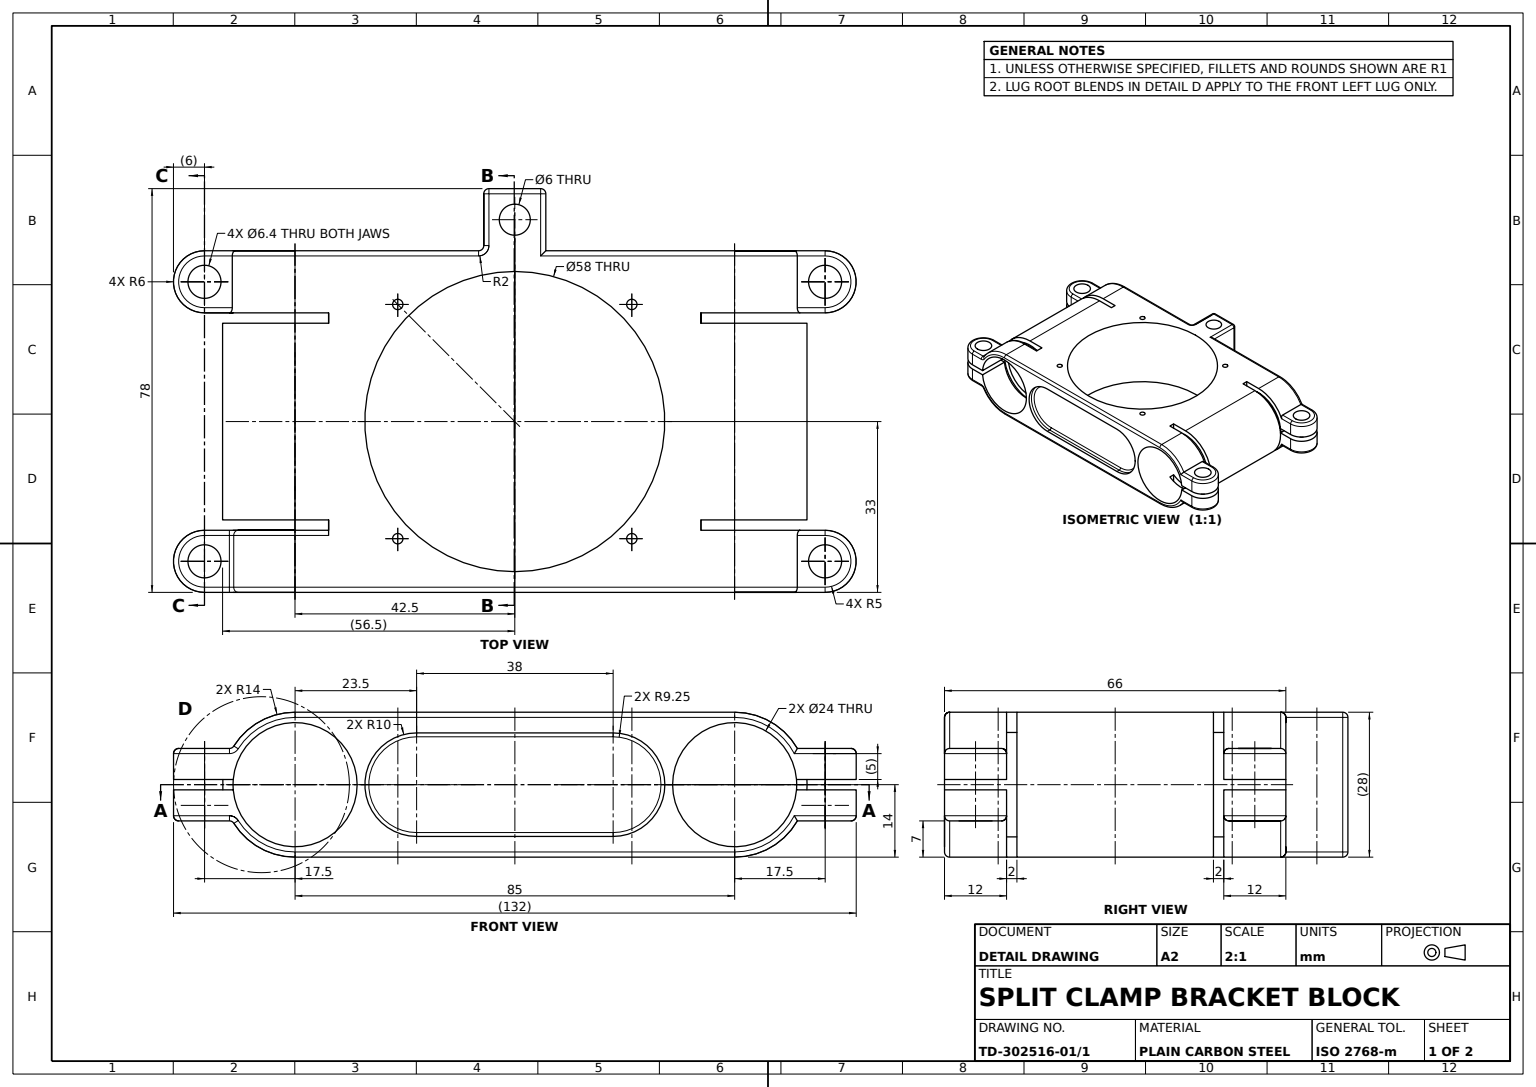
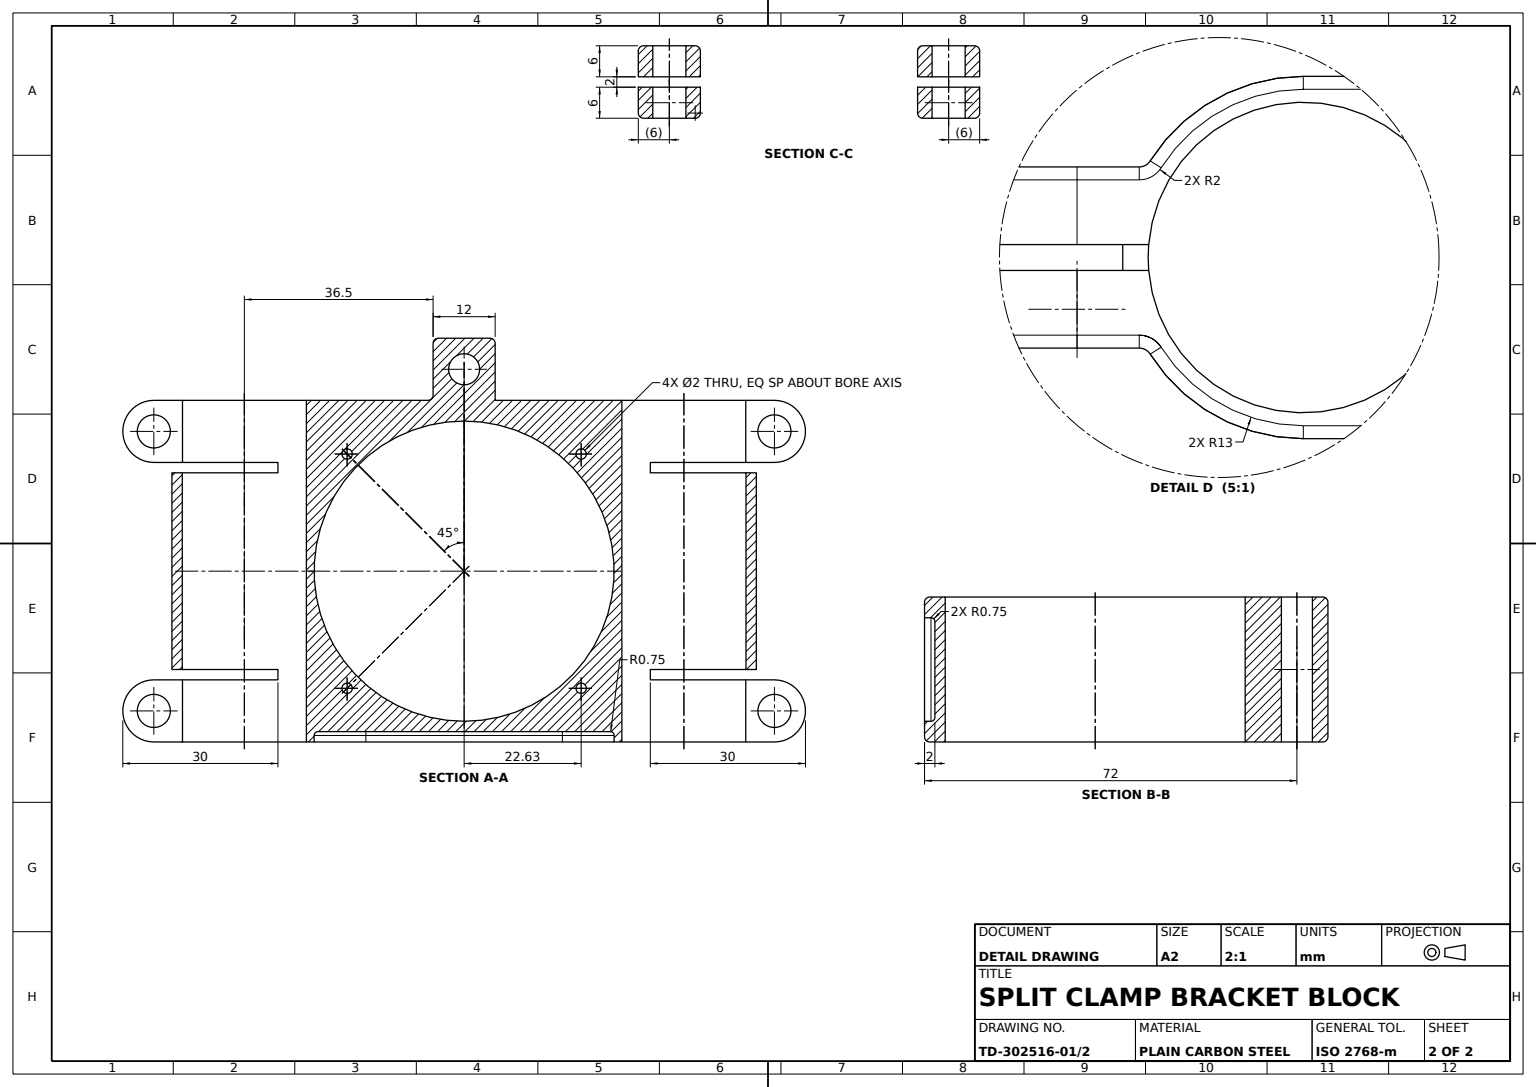
SolidWorks part; units mm, degrees
material "Plain Carbon Steel"
ref_plane "Front Plane" through (0, 0, 0) normal (0, 0, 1) x (1, 0, 0)
ref_plane "Top Plane" through (0, 0, 0) normal (0, 1, 0) x (1, 0, 0)
ref_plane "Right Plane" through (0, 0, 0) normal (1, 0, 0) x (0, 0, -1)
sketch "Body Profile Sketch" plane through (0, 0, 0) normal (0, 0, 1) x (1, 0, 0)
  line L0 (0, 0) -> (85, 0) construction
  line L1 (0, 14) -> (85, 14)
  line L2 (0, -14) -> (85, -14)
  arc A0 (0, 14) -> (0, -14) centre (0, 0) ccw
  arc A1 (85, -14) -> (85, 14) centre (85, 0) ccw
  point P3 (42.5, 0)
  dimension "D2" = 14
  dimension "D1" = 85
extrude "Carriage Body" add sketch "Body Profile Sketch" against normal blind 66
sketch "Rod Bore A Sketch" plane through (0, 0, 0) normal (0, 0, 1) x (1, 0, 0)
  circle A0 centre (0, 0) radius 12
  circle A1 centre (85, 0) radius 12
  dimension "D1" = 24
extrude "Rod Bore A Ø24" cut sketch "Rod Bore A Sketch" against normal blind 66
sketch "Side Pocket Sketch" plane through (0, 0, 0) normal (0, 0, 1) x (1, 0, 0)
  line L0 (23.5, 0) -> (61.5, 0) construction
  line L1 (23.5, 10) -> (61.5, 10)
  line L2 (23.5, -10) -> (61.5, -10)
  line L3 (85, 12) -> (85, 0) construction
  arc A0 (23.5, 10) -> (23.5, -10) centre (23.5, 0) ccw
  arc A1 (61.5, -10) -> (61.5, 10) centre (61.5, 0) ccw
  circle A2 centre (85, 0) radius 12 construction
  point P3 (42.5, 0)
  dimension "D3" = 10
  dimension "D1" = 38
  dimension "D2" = 42.5
extrude "Side Pocket 2mm" cut sketch "Side Pocket Sketch" against normal blind 2
sketch "Centre Bore Sketch" plane through (0, 14, 0) normal (0, 1, 0) x (1, 0, 0)
  line L0 (-14, 66) -> (-14, 0) construction
  circle A0 centre (42.5, 33) radius 29
  dimension "D1" = 58
  dimension "D2" = 33
  dimension "D3" = 56.5
extrude "Centre Bore Ø58" cut sketch "Centre Bore Sketch" against normal through all
sketch "Bore Screw Holes Sketch" plane through (0, 14, 0) normal (0, 1, 0) x (1, 0, 0)
  line L0 (42.5, 33) -> (68.5238, 59.0238) construction
  circle A1 centre (65.1274, 55.6274) radius 1
  circle A2 centre (65.1274, 10.3726) radius 1
  circle A3 centre (19.8726, 10.3726) radius 1
  circle A4 centre (19.8726, 55.6274) radius 1
  dimension "D1" = 22.6274
  dimension "D3" = 2
  dimension "D2" = 45
  dimension "D5" = 22.6274
  dimension "D6" = 22.6274
  dimension "D7" = 22.6274
  dimension "D4" = 4
extrude "Bore Screw Holes 4xØ2" cut sketch "Bore Screw Holes Sketch" against normal through all
ref_plane "Plane1" through (0, 0, 0) normal (0, 1, 0) x (1, 0, 0)
sketch "Clamp Lug Sketch" plane through (0, 0, 0) normal (0, 1, 0) x (1, 0, 0)
  line L0 (85, 0) -> (0, 0) construction
  line L1 (102.5, 12) -> (96.5, 12)
  line L2 (96.5, 12) -> (96.5, 0)
  line L3 (85, 0) -> (99, 0) construction
  line L4 (96.5, 0) -> (102.5, 0)
  arc A0 (102.5, 0) -> (102.5, 12) centre (102.5, 6) ccw
  dimension "D1" = 12
  dimension "D2" = 17.5
  dimension "D3" = 6
  dimension "D4" = 6
extrude "Clamp Lug" add sketch "Clamp Lug Sketch" along normal mid plane 14
sketch "Lug Split Sketch" plane through (0, 0, 0) normal (0, 1, 0) x (1, 0, 0)
  line L0 (97.1244, 0) -> (102.5, 0) construction
  line L1 (102.5, 12) -> (97.1244, 12) construction
  line L2 (97.1244, 0) -> (102.5, 0)
  line L3 (102.5, 12) -> (97.1244, 12)
  line L4 (97.1244, 12) -> (92.1244, 12)
  line L5 (92.1244, 12) -> (92.1244, 0)
  line L6 (85, 0) -> (97.1244, 0) construction
  line L7 (92.1244, 0) -> (97.1244, 0)
  arc A0 (102.5, 0) -> (102.5, 12) centre (102.5, 6) ccw construction
  arc A1 (102.5, 0) -> (102.5, 12) centre (102.5, 6) ccw
  dimension "D1" = 5
extrude "Lug Split" cut sketch "Lug Split Sketch" against normal mid plane 2
sketch "Lug Hole Sketch" plane through (0, 7, 0) normal (0, 1, 0) x (1, 0, 0)
  circle A0 centre (102.5, 6) radius 3.2
  dimension "D1" = 6.4
extrude "Lug Hole Ø6.4" cut sketch "Lug Hole Sketch" against normal through all
ref_plane "Plane2" through (0, 0, -33) normal (0, 0, 1) x (1, 0, 0)
mirror "Lug Mirror Plane2" about plane through (0, 0, -33) normal (0, 0, 1) of "Lug Split", "Lug Hole Ø6.4", "Clamp Lug"
ref_plane "Plane4" through (42.5, 0, 0) normal (1, 0, 0) x (0, 0, -1)
mirror "Lug Mirror Plane4" about plane through (42.5, 0, 0) normal (1, 0, 0) of "Lug Split", "Lug Hole Ø6.4", "Clamp Lug"
mirror "Lug Pair Mirror Plane2" about plane through (0, 0, -33) normal (0, 0, 1) of "Clamp Lug", "Lug Split", "Lug Hole Ø6.4", "Lug Mirror Plane4"
sketch "Rod Bore B Sketch" plane through (0, 0, -66) normal (0, 0, -1) x (-1, 0, 0)
  circle A0 centre (-85, 0) radius 12
  circle A1 centre (0, 0) radius 12
  dimension "D1" = 24
extrude "Rod Bore B Ø24" cut sketch "Rod Bore B Sketch" against normal through all
sketch "Clamp Split Slots Sketch" plane through (0, 14, 0) normal (0, 1, 0) x (1, 0, 0)
  line L0 (105.7, 60) -> (102.5, 60) construction
  line L1 (108.5, 54) -> (78.5, 54)
  line L2 (108.5, 54) -> (108.5, 52)
  line L3 (108.5, 52) -> (78.5, 52)
  line L4 (78.5, 54) -> (78.5, 52)
  line L5 (-15.4, 33) -> (15.4, 33) construction
  line L6 (78.5, 12) -> (78.5, 14)
  line L7 (108.5, 12) -> (108.5, 14)
  line L8 (108.5, 14) -> (78.5, 14)
  line L9 (108.5, 12) -> (78.5, 12)
  line L10 (42.5, -15.4) -> (42.5, 15.4) construction
  line L11 (6.5, 12) -> (6.5, 14)
  line L12 (-23.5, 12) -> (6.5, 12)
  line L13 (-23.5, 14) -> (6.5, 14)
  line L14 (-23.5, 12) -> (-23.5, 14)
  line L15 (6.5, 54) -> (6.5, 52)
  line L16 (-23.5, 52) -> (6.5, 52)
  line L17 (-23.5, 54) -> (6.5, 54)
  line L18 (-23.5, 54) -> (-23.5, 52)
  circle A0 centre (102.5, 60) radius 3.2 construction
  point P9 (108.5, 53)
  dimension "D1" = 6
  dimension "D2" = 2
  dimension "D3" = 6
  dimension "D4" = 30
extrude "Clamp Split Slots" cut sketch "Clamp Split Slots Sketch" against normal through all
sketch "Side Tab Sketch" plane through (0, 14, 0) normal (0, 1, 0) x (1, 0, 0)
  line L0 (85, 66) -> (0, 66) construction
  line L1 (36.5, 66) -> (48.5, 66)
  line L2 (36.5, 66) -> (36.5, 78)
  line L3 (36.5, 78) -> (48.5, 78)
  line L4 (48.5, 66) -> (48.5, 78)
  dimension "D1" = 12
  dimension "D2" = 12
  dimension "D3" = 36.5
extrude "Side Tab" add sketch "Side Tab Sketch" against normal blind 28
sketch "Side Tab Hole Sketch" plane through (0, 14, 0) normal (0, 1, 0) x (1, 0, 0)
  circle A0 centre (42.5, 72) radius 3
  dimension "D1" = 6
  dimension "D2" = 42.5
  dimension "D3" = 72
extrude "Side Tab Hole Ø6" cut sketch "Side Tab Hole Sketch" against normal blind 28
fillet "Lug Edge Fillets R1" radius 1 51 edges at (92, 12.1244, -66) (92, -12.1244, -66) (108.5, 7, -60) (99.8122, 7, -66) (99.8122, 7, -54) (99.8122, -7, -66) (108.5, -7, -60) (99.8122, -7, -54) (66.75, 14, -66) (-7, -12.1244, 0) (-23.5, 7, -6) (-14.8122, 7, 0) (-14.8122, 7, -12) (-14.8122, -7, 0) (-23.5, -7, -6) (-14.8122, -7, -12) (-7, -12.1244, -66) (-23.5, -7, -60) (-14.8122, -7, -54) (-14.8122, -7, -66) (-14.8122, 7, -54) (-14.8122, 7, -66) (-23.5, 7, -60) (-7, 12.1244, -66) (42.5, 14, 0) (-7, -12.1244, -12) (-7, 12.1244, -12) (3.25, -14, -12) (3.25, 14, -12) (92, -12.1244, 0) (42.5, -14, 0) (66.75, -14, -66) (18.25, 14, -66) (36.5, -14, -72) (36.5, 0, -66) (42.5, -14, -78) (36.5, 0, -78) (48.5, -14, -72) (48.5, 0, -78) (36.5, 14, -72) (48.5, 14, -72) (42.5, 14, -78) (-7, 12.1244, 0) (92, 12.1244, 0) (108.5, -7, -6) (99.8122, -7, -12) (99.8122, -7, 0) (99.8122, 7, -12) (99.8122, 7, 0) (108.5, 7, -6) (18.25, -14, -66)
fillet "Side Pocket Fillet R0.75" radius 0.75 4 edges at (13.5, 0, -2) (42.5, 10, -2) (71.5, 0, -2) (42.5, -10, -2)
